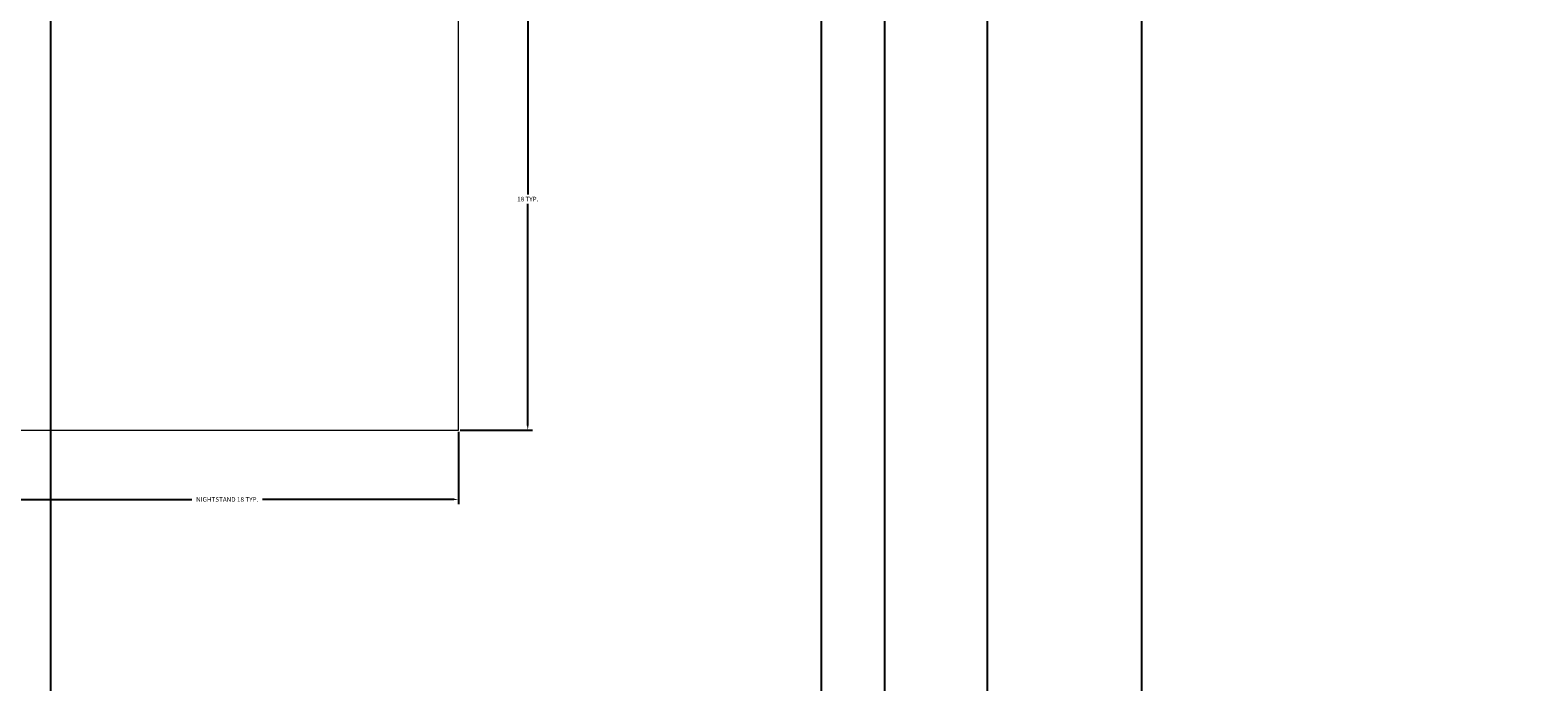
# Model space of a CAD drawing. Units: inches. Extents: x 2231 to 2461, y 2045 to 2455.
# Tile 53 of 95: x 2262 to 2320, y 2307 to 2333. Entities that reach past the tile are written whole.
import ezdxf

# ---------------------------------------------------------------- set-up
doc = ezdxf.new("R2010")
doc.units = ezdxf.units.IN
doc.layers.add('A-ANNO-DIMS', color=2, linetype='Continuous', lineweight=18)
doc.layers.add('A-FURN', color=9, linetype='Continuous', lineweight=18)
doc.styles.get("Standard").update_dxf_attribs({"font": 'arial.ttf'})
doc.dimstyles.get("Standard").update_dxf_attribs({"dimtxt": 0.18, "dimasz": 0.18, "dimexe": 0.18, "dimexo": 0.0625, "dimgap": 0.09, "dimtad": 0, "dimtih": 1, "dimtoh": 1, "dimdec": 4, "dimzin": 0, "dimdsep": 46, "dimtxsty": 'Standard', "dimcen": 0.09, "dimadec": 0, "dimazin": 0, "dimtfac": 1, "dimtdec": 4, "dimtofl": 0, "dimtmove": 0, "dimatfit": 3, "dimfxl": 1, "dimtolj": 1, "dimtzin": 0, "dimarcsym": 0})

# ---------------------------------------------------------------- blocks, each defined once
blk = doc.blocks.new('NIGHTSTAND-18IN')
blk.add_lwpolyline([(0, 0), (18, 0), (18, 18), (0, 18)], close=True)
blk = doc.blocks.new('*D17')
at = {"layer": 'A-ANNO-DIMS', "color": 0, "lineweight": -2, "transparency": 16777216}
for p, q in [((2260.188, 2317.191), (2260.188, 2314.373)), ((2278.188, 2317.191), (2278.188, 2314.373)), ((2260.368, 2314.553), (2267.812, 2314.553)), ((2278.008, 2314.553), (2270.564, 2314.553))]:
    blk.add_line(p, q, dxfattribs=at)
at = {"layer": 'A-ANNO-DIMS', "color": 0, "transparency": 16777216}
for points in [[(2260.368, 2314.583), (2260.368, 2314.523), (2260.188, 2314.553)], [(2278.008, 2314.583), (2278.008, 2314.523), (2278.188, 2314.553)]]:
    blk.add_solid(points, dxfattribs=at)
at = {"layer": 'Defpoints', "color": 0, "transparency": 16777216}
for p in [(2260.188, 2317.253), (2278.188, 2317.253), (2278.188, 2314.553)]:
    blk.add_point(p, dxfattribs=at)
at = {"layer": 'A-ANNO-DIMS', "color": 0, "transparency": 16777216, "insert": (2269.188, 2314.553), "char_height": 0.18, "attachment_point": 5}
blk.add_mtext('\\A1;NIGHTSTAND 18 TYP.', dxfattribs=at)
blk = doc.blocks.new('*D18')
at = {"layer": 'A-ANNO-DIMS', "color": 0, "lineweight": -2, "transparency": 16777216}
for p, q in [((2278.251, 2335.253), (2281.068, 2335.253)), ((2280.888, 2335.073), (2280.888, 2326.435)), ((2280.888, 2317.433), (2280.888, 2326.071)), ((2278.251, 2317.253), (2281.068, 2317.253))]:
    blk.add_line(p, q, dxfattribs=at)
at = {"layer": 'A-ANNO-DIMS', "color": 0, "transparency": 16777216}
for points in [[(2280.858, 2335.073), (2280.918, 2335.073), (2280.888, 2335.253)], [(2280.858, 2317.433), (2280.918, 2317.433), (2280.888, 2317.253)]]:
    blk.add_solid(points, dxfattribs=at)
at = {"layer": 'Defpoints', "color": 0, "transparency": 16777216}
for p in [(2278.188, 2335.253), (2280.888, 2335.253), (2278.188, 2317.253)]:
    blk.add_point(p, dxfattribs=at)
at = {"layer": 'A-ANNO-DIMS', "color": 0, "transparency": 16777216, "insert": (2280.888, 2326.253), "char_height": 0.18, "attachment_point": 5}
blk.add_mtext('\\A1;18 TYP.', dxfattribs=at)
blk = doc.blocks.new('*D47')
at = {"layer": 'A-ANNO-DIMS', "color": 0, "lineweight": -2, "transparency": 16777216}
for p, q in [((2258.794, 2182.895), (2258.794, 2454.645)), ((2258.974, 2454.465), (2276.575, 2454.465)), ((2294.614, 2454.465), (2277.012, 2454.465)), ((2294.794, 2182.895), (2294.794, 2454.645))]:
    blk.add_line(p, q, dxfattribs=at)
at = {"layer": 'A-ANNO-DIMS', "color": 0, "transparency": 16777216}
for points in [[(2258.974, 2454.495), (2258.974, 2454.435), (2258.794, 2454.465)], [(2294.614, 2454.495), (2294.614, 2454.435), (2294.794, 2454.465)]]:
    blk.add_solid(points, dxfattribs=at)
at = {"layer": 'Defpoints', "color": 0, "transparency": 16777216}
for p in [(2294.794, 2454.465), (2258.794, 2182.833), (2294.794, 2182.833)]:
    blk.add_point(p, dxfattribs=at)
at = {"layer": 'A-ANNO-DIMS', "color": 0, "transparency": 16777216, "insert": (2276.794, 2454.465), "char_height": 0.18, "attachment_point": 5}
blk.add_mtext('\\A1;36', dxfattribs=at)
blk = doc.blocks.new('*D49')
at = {"layer": 'A-ANNO-DIMS', "color": 0, "lineweight": -2, "transparency": 16777216}
for p, q in [((2298.794, 2182.895), (2298.794, 2454.645)), ((2298.974, 2454.465), (2301.644, 2454.465)), ((2304.614, 2454.465), (2301.943, 2454.465)), ((2304.794, 2182.895), (2304.794, 2454.645))]:
    blk.add_line(p, q, dxfattribs=at)
at = {"layer": 'A-ANNO-DIMS', "color": 0, "transparency": 16777216}
for points in [[(2298.974, 2454.495), (2298.974, 2454.435), (2298.794, 2454.465)], [(2304.614, 2454.495), (2304.614, 2454.435), (2304.794, 2454.465)]]:
    blk.add_solid(points, dxfattribs=at)
at = {"layer": 'Defpoints', "color": 0, "transparency": 16777216}
for p in [(2304.794, 2454.465), (2298.794, 2182.833), (2304.794, 2182.833)]:
    blk.add_point(p, dxfattribs=at)
at = {"layer": 'A-ANNO-DIMS', "color": 0, "transparency": 16777216, "insert": (2301.794, 2454.465), "char_height": 0.18, "attachment_point": 5}
blk.add_mtext('\\A1;6', dxfattribs=at)
blk = doc.blocks.new('*D50')
at = {"layer": 'A-ANNO-DIMS', "color": 0, "lineweight": -2, "transparency": 16777216}
for p, q in [((2304.794, 2182.895), (2304.794, 2454.645)), ((2304.974, 2454.465), (2319.575, 2454.465)), ((2334.614, 2454.465), (2320.012, 2454.465)), ((2334.794, 2182.895), (2334.794, 2454.645))]:
    blk.add_line(p, q, dxfattribs=at)
at = {"layer": 'A-ANNO-DIMS', "color": 0, "transparency": 16777216}
for points in [[(2304.974, 2454.495), (2304.974, 2454.435), (2304.794, 2454.465)], [(2334.614, 2454.495), (2334.614, 2454.435), (2334.794, 2454.465)]]:
    blk.add_solid(points, dxfattribs=at)
at = {"layer": 'Defpoints', "color": 0, "transparency": 16777216}
for p in [(2334.794, 2454.465), (2304.794, 2182.833), (2334.794, 2182.833)]:
    blk.add_point(p, dxfattribs=at)
at = {"layer": 'A-ANNO-DIMS', "color": 0, "transparency": 16777216, "insert": (2319.794, 2454.465), "char_height": 0.18, "attachment_point": 5}
blk.add_mtext('\\A1;30', dxfattribs=at)
blk = doc.blocks.new('*D62')
at = {"layer": 'A-ANNO-DIMS', "color": 0, "lineweight": -2, "transparency": 16777216}
for p, q in [((2262.321, 2255.176), (2262.321, 2454.645)), ((2262.501, 2454.465), (2277.102, 2454.465)), ((2292.141, 2454.465), (2277.539, 2454.465)), ((2292.321, 2253.176), (2292.321, 2454.645))]:
    blk.add_line(p, q, dxfattribs=at)
at = {"layer": 'A-ANNO-DIMS', "color": 0, "transparency": 16777216}
for points in [[(2262.501, 2454.495), (2262.501, 2454.435), (2262.321, 2454.465)], [(2292.141, 2454.495), (2292.141, 2454.435), (2292.321, 2454.465)]]:
    blk.add_solid(points, dxfattribs=at)
at = {"layer": 'Defpoints', "color": 0, "transparency": 16777216}
for p in [(2292.321, 2454.465), (2262.321, 2255.114), (2292.321, 2253.114)]:
    blk.add_point(p, dxfattribs=at)
at = {"layer": 'A-ANNO-DIMS', "color": 0, "transparency": 16777216, "insert": (2277.321, 2454.465), "char_height": 0.18, "attachment_point": 5}
blk.add_mtext('\\A1;30', dxfattribs=at)

msp = doc.modelspace()

# ---------------------------------------------------------------- block references
at = {"layer": 'A-FURN'}
msp.add_blockref('NIGHTSTAND-18IN', (2260.188, 2317.253), dxfattribs=at)

# ---------------------------------------------------------------- dimensions: what is measured, and where the dimension line sits
at = {"layer": 'A-ANNO-DIMS'}
for base, p1, p2, picture, middle in [((2294.7935, 2454.4653), (2258.7935, 2182.8328), (2294.7935, 2182.8328), '*D47', (2276.7935, 2454.4653)), ((2292.3207, 2454.4653), (2262.3207, 2255.1137), (2292.3207, 2253.1137), '*D62', (2277.3207, 2454.4653)), ((2304.7935, 2454.4653), (2298.7935, 2182.8328), (2304.7935, 2182.8328), '*D49', (2301.7935, 2454.4653)), ((2334.7935, 2454.4653), (2304.7935, 2182.8328), (2334.7935, 2182.8328), '*D50', (2319.7935, 2454.4653))]:
    dim = msp.add_linear_dim(base=base, p1=p1, p2=p2, dimstyle='Standard', override={"dimdec": 0, "dimlfac": 1, "dimrnd": 0, "dimzin": 0, "dimdsep": 46, "dimlunit": 2}, dxfattribs=at)
    dim.commit()
    dim.dimension.update_dxf_attribs({"geometry": picture, "text_midpoint": middle})
dim = msp.add_linear_dim(base=(2280.8881, 2335.2534), p1=(2278.1881, 2317.2534), p2=(2278.1881, 2335.2534), angle=90, text='<> TYP.', dimstyle='Standard', override={"dimdec": 0, "dimlfac": 1, "dimrnd": 0, "dimzin": 0, "dimdsep": 46, "dimlunit": 2}, dxfattribs=at)
dim.commit()
dim.dimension.update_dxf_attribs({"geometry": '*D18', "text_midpoint": (2280.8881, 2326.2534)})
dim = msp.add_linear_dim(base=(2278.1881, 2314.5534), p1=(2260.1881, 2317.2534), p2=(2278.1881, 2317.2534), text='NIGHTSTAND <> TYP.', dimstyle='Standard', override={"dimdec": 0, "dimlfac": 1, "dimrnd": 0, "dimzin": 0, "dimdsep": 46, "dimlunit": 2}, dxfattribs=at)
dim.commit()
dim.dimension.update_dxf_attribs({"geometry": '*D17', "text_midpoint": (2269.1881, 2314.5534)})

doc.saveas('drawing.dxf')
